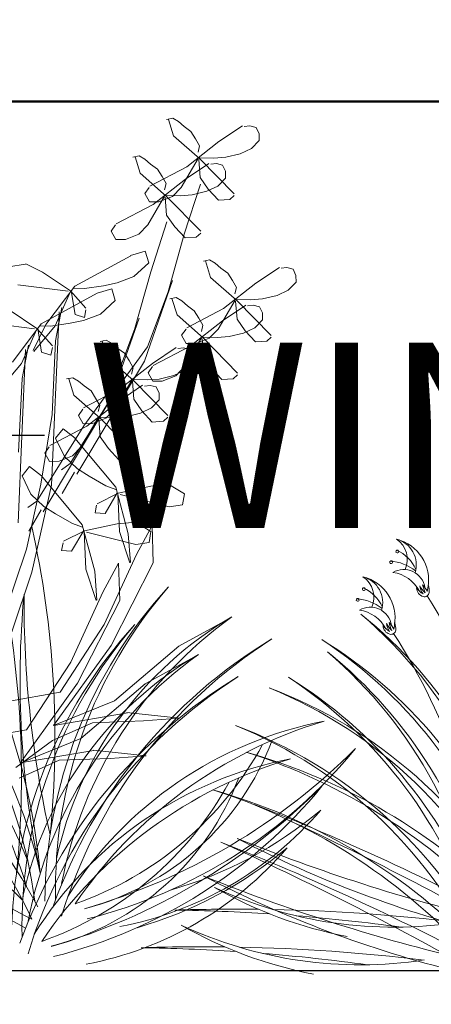
# Model space of a CAD drawing. Units: inches. Extents: x 89 to 490, y -59 to 378.
# Tile 9 of 20: x 339 to 352, y -24 to 7. Entities that reach past the tile are written whole.
import ezdxf

# ---------------------------------------------------------------- set-up
doc = ezdxf.new("R2010")
doc.units = ezdxf.units.IN
doc.header["$MEASUREMENT"] = 0
for name, color, linetype, lineweight in [('A-ANNO-DIMS', 2, 'Continuous', 18), ('L-PLNT', 94, 'Continuous', 18), ('L-PLNT-EDGE', 31, 'Continuous', 25), ('Outer Walls', 12, 'Continuous', 50), ('Windows', 171, 'Continuous', 25)]:
    doc.layers.add(name, color=color, linetype=linetype, lineweight=lineweight)
doc.layers.add('fl', color=73, linetype='Continuous', lineweight=9, true_color=0xa3d166)
doc.styles.get("Standard").update_dxf_attribs({"font": 'arial.ttf'})
doc.dimstyles.get("Standard").update_dxf_attribs({"dimtxt": 6, "dimasz": 4, "dimexe": 3, "dimexo": 3, "dimgap": 0.09, "dimtad": 0, "dimtih": 1, "dimtoh": 1, "dimdec": 1, "dimzin": 0, "dimdsep": 46, "dimlunit": 3, "dimtxsty": 'Standard', "dimcen": 0.09, "dimadec": 0, "dimazin": 0, "dimtfac": 1, "dimtdec": 1, "dimtofl": 0, "dimtmove": 0, "dimatfit": 3, "dimfxl": 1, "dimtolj": 1, "dimtzin": 0, "dimarcsym": 0})

# ---------------------------------------------------------------- blocks, each defined once
blk = doc.blocks.new('Window')
blk.add_lwpolyline([(588.369, 99.053), (588.369, 90.053), (516.369, 90.053), (516.369, 99.053)], close=True)
blk = doc.blocks.new('Plantation')
at = {"layer": 'fl'}
for p, q in [((567.452, 39.025), (567.652, 39.065)), ((567.52, 39.031), (567.683, 38.502)), ((567.652, 39.065), (567.835, 38.959)), ((567.835, 38.959), (568.02, 38.798)), ((568.02, 38.798), (568.241, 38.638)), ((568.241, 38.638), (568.391, 38.404)), ((569.148, 38.309), (569.909, 38.821)), ((570.148, 38.817), (569.967, 38.796)), ((570.349, 38.766), (570.148, 38.817)), ((570.444, 38.567), (570.349, 38.766)), ((570.448, 38.349), (570.444, 38.567)), ((567.683, 38.502), (568.535, 37.754)), ((568.107, 37.496), (569.148, 38.309)), ((568.391, 38.404), (568.522, 38.17)), ((570.198, 38.09), (570.448, 38.349)), ((568.522, 38.17), (568.471, 37.969)), ((569.366, 37.802), (569.837, 37.92)), ((569.837, 37.92), (570.198, 38.09)), ((566.368, 37.807), (566.568, 37.847)), ((566.436, 37.813), (566.6, 37.284)), ((566.568, 37.847), (566.752, 37.741)), ((566.752, 37.741), (566.936, 37.58)), ((567.927, 36.83), (568.475, 37.768)), ((568.065, 37.091), (568.825, 37.603)), ((568.494, 37.732), (568.54, 37.15)), ((568.529, 37.788), (568.984, 37.777)), ((568.535, 37.754), (569.643, 36.625)), ((569.065, 37.599), (568.883, 37.578)), ((568.984, 37.777), (569.366, 37.802)), ((569.266, 37.548), (569.065, 37.599)), ((566.6, 37.284), (567.452, 36.536)), ((566.913, 36.872), (568.107, 37.496)), ((566.936, 37.58), (567.157, 37.42)), ((567.157, 37.42), (567.307, 37.186)), ((569.36, 37.349), (569.266, 37.548)), ((569.364, 37.131), (569.36, 37.349)), ((567.023, 36.278), (568.065, 37.091)), ((567.307, 37.186), (567.439, 36.952)), ((568.54, 37.15), (568.801, 36.773)), ((569.114, 36.872), (569.364, 37.131)), ((566.89, 36.83), (566.748, 36.627)), ((567.439, 36.952), (567.387, 36.751)), ((567.641, 36.534), (567.927, 36.83)), ((568.024, 35.31), (568.552, 36.932)), ((568.282, 36.584), (568.753, 36.702)), ((568.753, 36.702), (569.114, 36.872)), ((568.801, 36.773), (569.135, 36.414)), ((566.748, 36.627), (566.898, 36.357)), ((566.843, 35.612), (567.391, 36.55)), ((566.898, 36.357), (567.208, 36.362)), ((567.208, 36.362), (567.641, 36.534)), ((567.41, 36.514), (567.456, 35.932)), ((567.445, 36.57), (567.9, 36.559)), ((567.452, 36.536), (568.56, 35.407)), ((567.9, 36.559), (568.282, 36.584)), ((569.135, 36.414), (569.499, 36.439)), ((569.499, 36.439), (569.642, 36.569)), ((565.829, 35.654), (567.023, 36.278)), ((566.94, 34.092), (567.468, 35.714)), ((567.456, 35.932), (567.718, 35.555)), ((565.806, 35.612), (565.664, 35.409)), ((565.664, 35.409), (565.815, 35.139)), ((566.557, 35.316), (566.843, 35.612)), ((567.718, 35.555), (568.051, 35.196)), ((565.815, 35.139), (566.124, 35.144)), ((566.124, 35.144), (566.557, 35.316)), ((567.504, 33.445), (568.024, 35.31)), ((568.051, 35.196), (568.415, 35.221)), ((568.415, 35.221), (568.558, 35.351)), ((566.767, 34.761), (566.292, 34.62)), ((566.88, 34.391), (566.767, 34.761)), ((564.484, 33.634), (566.297, 34.619)), ((568.645, 34.441), (568.845, 34.481)), ((568.713, 34.447), (568.877, 33.918)), ((568.845, 34.481), (569.029, 34.375)), ((562.897, 34.348), (562.341, 34.259)), ((562.903, 34.358), (563.447, 34.084)), ((566.397, 33.944), (566.88, 34.391)), ((566.42, 32.227), (566.94, 34.092)), ((569.029, 34.375), (569.213, 34.214)), ((569.213, 34.214), (569.435, 34.054)), ((570.342, 33.725), (571.102, 34.237)), ((571.342, 34.233), (571.16, 34.212)), ((571.543, 34.182), (571.342, 34.233)), ((571.637, 33.983), (571.543, 34.182)), ((563.447, 34.084), (564.343, 33.483)), ((565.856, 33.736), (566.397, 33.944)), ((566.737, 31.205), (567.647, 33.818)), ((568.877, 33.918), (569.729, 33.169)), ((569.435, 34.054), (569.584, 33.82)), ((569.584, 33.82), (569.716, 33.586)), ((571.641, 33.765), (571.637, 33.983)), ((562.643, 33.679), (564.267, 33.469)), ((563.554, 32.387), (564.484, 33.634)), ((563.848, 32.345), (564.347, 33.457)), ((564.343, 33.483), (564.848, 32.917)), ((564.493, 32.715), (564.373, 33.484)), ((564.451, 33.565), (564.797, 33.558)), ((564.797, 33.558), (565.419, 33.648)), ((565.683, 33.543), (565.208, 33.402)), ((565.419, 33.648), (565.856, 33.736)), ((565.796, 33.173), (565.683, 33.543)), ((569.3, 32.912), (570.342, 33.725)), ((569.716, 33.586), (569.665, 33.384)), ((571.03, 33.335), (571.391, 33.505)), ((571.391, 33.505), (571.641, 33.765)), ((563.4, 32.416), (565.213, 33.401)), ((565.313, 32.726), (565.796, 33.173)), ((566.835, 31.672), (567.504, 33.445)), ((567.562, 33.223), (567.761, 33.263)), ((567.629, 33.229), (567.793, 32.7)), ((567.761, 33.263), (567.945, 33.157)), ((567.945, 33.157), (568.13, 32.996)), ((569.12, 32.246), (569.668, 33.184)), ((569.687, 33.148), (569.733, 32.566)), ((569.722, 33.203), (570.177, 33.193)), ((569.729, 33.169), (570.837, 32.04)), ((570.177, 33.193), (570.559, 33.218)), ((570.559, 33.218), (571.03, 33.335)), ((562.363, 32.866), (563.259, 32.265)), ((563.863, 31.862), (564.07, 32.939)), ((564.848, 32.868), (564.8, 32.614)), ((568.106, 32.288), (569.3, 32.912)), ((568.13, 32.996), (568.351, 32.836)), ((568.351, 32.836), (568.5, 32.602)), ((569.258, 32.507), (570.018, 33.019)), ((570.258, 33.015), (570.076, 32.994)), ((570.459, 32.964), (570.258, 33.015)), ((570.553, 32.765), (570.459, 32.964)), ((563.978, 32.797), (563.734, 27.189)), ((564.335, 32.43), (564.772, 32.518)), ((564.8, 32.614), (564.493, 32.715)), ((564.772, 32.518), (565.313, 32.726)), ((565.653, 29.987), (566.564, 32.6)), ((567.793, 32.7), (568.645, 31.951)), ((568.216, 31.694), (569.258, 32.507)), ((568.5, 32.602), (568.632, 32.367)), ((569.733, 32.566), (569.995, 32.188)), ((570.307, 32.287), (570.557, 32.547)), ((570.557, 32.547), (570.553, 32.765)), ((561.559, 32.461), (563.183, 32.251)), ((562.47, 31.169), (563.4, 32.416)), ((562.765, 31.127), (563.263, 32.239)), ((563.145, 31.546), (563.554, 32.387)), ((563.159, 31.523), (563.848, 32.345)), ((563.259, 32.265), (563.764, 31.699)), ((563.409, 31.497), (563.289, 32.266)), ((563.367, 32.347), (563.713, 32.34)), ((563.713, 32.34), (564.335, 32.43)), ((565.751, 30.454), (566.42, 32.227)), ((568.083, 32.246), (567.941, 32.043)), ((568.632, 32.367), (568.581, 32.166)), ((568.834, 31.95), (569.12, 32.246)), ((569.946, 32.117), (570.307, 32.287)), ((569.995, 32.188), (570.328, 31.83)), ((563.75, 29.477), (563.863, 31.862)), ((565.306, 31.847), (565.506, 31.887)), ((565.506, 31.887), (565.69, 31.781)), ((567.941, 32.043), (568.092, 31.773)), ((568.037, 31.028), (568.584, 31.966)), ((568.401, 31.778), (568.834, 31.95)), ((568.603, 31.93), (568.65, 31.348)), ((568.638, 31.985), (569.093, 31.975)), ((568.645, 31.951), (569.753, 30.822)), ((569.093, 31.975), (569.475, 32)), ((569.475, 32), (569.946, 32.117)), ((570.692, 31.855), (570.835, 31.984)), ((562.894, 31.579), (562.65, 25.971)), ((562.78, 30.644), (562.986, 31.721)), ((563.765, 31.65), (563.716, 31.396)), ((565.374, 31.853), (565.537, 31.324)), ((565.69, 31.781), (565.874, 31.62)), ((565.86, 30.326), (566.835, 31.672)), ((565.874, 31.62), (566.095, 31.46)), ((567.002, 31.131), (567.763, 31.643)), ((567.022, 31.07), (568.216, 31.694)), ((568.002, 31.639), (567.821, 31.618)), ((568.203, 31.588), (568.002, 31.639)), ((568.092, 31.773), (568.401, 31.778)), ((568.298, 31.389), (568.203, 31.588)), ((570.328, 31.83), (570.692, 31.855)), ((563.716, 31.396), (563.409, 31.497)), ((565.537, 31.324), (566.389, 30.575)), ((566.095, 31.46), (566.245, 31.226)), ((566.245, 31.226), (566.376, 30.992)), ((568.302, 31.171), (568.298, 31.389)), ((568.65, 31.348), (568.911, 30.97)), ((562.075, 30.305), (562.765, 31.127)), ((564.547, 27.545), (566.737, 31.205)), ((565.961, 30.318), (567.002, 31.131)), ((566.376, 30.992), (566.325, 30.79)), ((567, 31.028), (566.858, 30.825)), ((567.691, 30.741), (568.052, 30.912)), ((567.751, 30.732), (568.037, 31.028)), ((568.052, 30.912), (568.302, 31.171)), ((568.911, 30.97), (569.245, 30.612)), ((562.666, 28.259), (562.78, 30.644)), ((564.222, 30.629), (564.422, 30.669)), ((564.29, 30.635), (564.454, 30.106)), ((564.422, 30.669), (564.606, 30.563)), ((565.781, 29.652), (566.329, 30.59)), ((566.383, 30.609), (566.838, 30.599)), ((566.838, 30.599), (567.22, 30.624)), ((566.858, 30.825), (567.008, 30.555)), ((567.22, 30.624), (567.691, 30.741)), ((567.317, 30.56), (567.751, 30.732)), ((569.245, 30.612), (569.608, 30.637)), ((569.608, 30.637), (569.751, 30.766)), ((564.339, 27.892), (565.86, 30.326)), ((564.606, 30.563), (564.79, 30.402)), ((564.767, 29.694), (565.961, 30.318)), ((564.776, 29.108), (565.751, 30.454)), ((564.79, 30.402), (565.012, 30.242)), ((565.919, 29.913), (566.679, 30.425)), ((566.348, 30.554), (566.394, 29.972)), ((566.389, 30.575), (567.497, 29.447)), ((566.919, 30.421), (566.737, 30.4)), ((567.12, 30.37), (566.919, 30.421)), ((567.008, 30.555), (567.317, 30.56)), ((567.214, 30.171), (567.12, 30.37)), ((563.463, 26.327), (565.653, 29.987)), ((564.454, 30.106), (565.306, 29.357)), ((565.012, 30.242), (565.161, 30.008)), ((565.161, 30.008), (565.293, 29.774)), ((566.394, 29.972), (566.656, 29.594)), ((566.968, 29.694), (567.218, 29.953)), ((567.218, 29.953), (567.214, 30.171)), ((564.744, 29.652), (564.602, 29.449)), ((564.877, 29.1), (565.919, 29.913)), ((565.293, 29.774), (565.242, 29.572)), ((565.495, 29.356), (565.781, 29.652)), ((566.607, 29.523), (566.968, 29.694)), ((563.389, 27.228), (563.75, 29.477)), ((564.602, 29.449), (564.753, 29.179)), ((564.697, 28.434), (565.245, 29.372)), ((565.062, 29.184), (565.495, 29.356)), ((565.264, 29.336), (565.31, 28.754)), ((565.299, 29.391), (565.754, 29.381)), ((565.306, 29.357), (566.414, 28.229)), ((565.754, 29.381), (566.136, 29.406)), ((566.136, 29.406), (566.607, 29.523)), ((566.656, 29.594), (566.989, 29.236)), ((567.353, 29.261), (567.496, 29.391)), ((563.255, 26.674), (564.776, 29.108)), ((563.683, 28.476), (564.877, 29.1)), ((563.864, 28.713), (564.105, 29.016)), ((564.105, 29.016), (564.495, 28.709)), ((564.753, 29.179), (565.062, 29.184)), ((566.989, 29.236), (567.353, 29.261)), ((564.148, 28.119), (563.864, 28.713)), ((565.812, 27.125), (564.489, 28.71)), ((565.31, 28.754), (565.572, 28.376)), ((563.66, 28.434), (563.518, 28.231)), ((564.412, 28.138), (564.697, 28.434)), ((565.572, 28.376), (565.905, 28.018)), ((563.518, 28.231), (563.669, 27.961)), ((563.978, 27.966), (564.412, 28.138)), ((564.574, 27.726), (564.148, 28.119)), ((565.905, 28.018), (566.269, 28.043)), ((566.269, 28.043), (566.412, 28.173)), ((562.78, 27.495), (563.021, 27.798)), ((563.021, 27.798), (563.411, 27.491)), ((563.669, 27.961), (563.978, 27.966)), ((564.054, 27.688), (564.339, 27.892)), ((564.948, 27.484), (564.574, 27.726)), ((563.064, 26.901), (562.78, 27.495)), ((564.728, 25.907), (563.405, 27.492)), ((564.08, 26.921), (564.478, 27.612)), ((565.493, 27.17), (564.948, 27.484)), ((562.927, 25.122), (563.389, 27.228)), ((563.734, 27.189), (563.1, 24.376)), ((565.817, 27.05), (565.493, 27.17)), ((566.216, 25.623), (565.812, 27.125)), ((566.941, 27.162), (565.887, 26.933)), ((567.548, 27.216), (566.941, 27.162)), ((567.55, 27.205), (568.034, 26.917)), ((563.49, 26.508), (563.064, 26.901)), ((565.887, 26.933), (565.209, 26.594)), ((565.465, 26.275), (565.86, 26.945)), ((565.927, 25.693), (565.874, 26.911)), ((567.539, 26.49), (565.952, 26.892)), ((568.034, 26.917), (567.97, 26.555)), ((562.97, 26.47), (563.255, 26.674)), ((563.864, 26.266), (563.49, 26.508)), ((565.19, 26.548), (565.142, 26.294)), ((567.97, 26.555), (567.539, 26.49)), ((562.996, 25.703), (563.394, 26.394)), ((564.409, 25.952), (563.864, 26.266)), ((565.142, 26.294), (565.465, 26.275)), ((564.733, 25.832), (564.409, 25.952)), ((565.133, 24.405), (564.728, 25.907)), ((565.858, 25.944), (564.803, 25.715)), ((566.464, 25.998), (565.858, 25.944)), ((566.466, 25.987), (566.95, 25.699)), ((566.481, 24.951), (566.984, 25.892)), ((566.984, 25.892), (567.025, 24.678)), ((564.803, 25.715), (564.125, 25.376)), ((564.381, 25.057), (564.776, 25.727)), ((564.844, 24.475), (564.79, 25.693)), ((566.456, 25.272), (564.869, 25.674)), ((566.265, 24.675), (565.927, 25.693)), ((566.287, 24.692), (566.216, 25.623)), ((566.95, 25.699), (566.886, 25.337)), ((564.106, 25.33), (564.058, 25.076)), ((566.886, 25.337), (566.456, 25.272)), ((562.176, 22.909), (562.927, 25.122)), ((564.058, 25.076), (564.381, 25.057)), ((565.44, 22.68), (566.481, 24.951)), ((565.397, 23.733), (565.9, 24.674)), ((567.025, 24.678), (565.658, 22.007)), ((565.9, 24.674), (565.941, 23.46)), ((563.1, 24.376), (562.451, 22.451)), ((565.181, 23.457), (564.844, 24.475)), ((565.203, 23.474), (565.133, 24.405)), ((564.357, 21.462), (565.397, 23.733)), ((565.941, 23.46), (564.574, 20.789)), ((564.008, 20.492), (565.44, 22.68)), ((567.846, 21.984), (569.564, 22.918)), ((565.658, 22.007), (563.802, 19.415)), ((565.768, 20.212), (567.846, 21.984)), ((566.762, 20.766), (568.481, 21.7)), ((562.924, 19.274), (564.357, 21.462)), ((564.574, 20.789), (562.718, 18.197)), ((564.684, 18.994), (566.762, 20.766)), ((562.317, 20.191), (564.008, 20.492)), ((563.802, 19.415), (565.768, 20.212)), ((566.19, 19.825), (563.803, 19.421)), ((566.169, 19.836), (567.877, 19.652)), ((565.063, 19.507), (563.77, 18.928)), ((566.713, 19.563), (565.063, 19.507)), ((567.877, 19.652), (566.713, 19.563)), ((561.233, 18.973), (562.924, 19.274)), ((563.77, 18.928), (562.584, 18.061)), ((562.718, 18.197), (564.684, 18.994)), ((565.106, 18.607), (562.719, 18.203)), ((565.086, 18.618), (566.793, 18.434)), ((563.979, 18.289), (562.686, 17.71)), ((565.63, 18.345), (563.979, 18.289)), ((566.793, 18.434), (565.63, 18.345))]:
    blk.add_line(p, q, dxfattribs=at)
for centre, radius, start, end in [((532.353, 19.019), 31.492, 354.2791, 12.5427), ((574.665, 24.613), 0.863, 342.816, 75.0201), ((574.448, 24.787), 0.793, 335.7976, 56.2278), ((574.561, 24.118), 1.368, 349.633, 76.1366), ((574.916, 25.045), 0.0459, 19.649, 199.649), ((574.916, 25.045), 0.0459, 199.649, 19.649), ((574.381, 23.96), 1.243, 24.0842, 65.3008), ((531.269, 17.801), 31.492, 354.2791, 12.5427), ((574.717, 24.698), 0.0459, 19.649, 199.649), ((574.717, 24.698), 0.0459, 199.649, 19.649), ((574.622, 23.348), 1.386, 50.416, 87.3549), ((573.582, 23.395), 0.863, 342.816, 75.0201), ((573.364, 23.569), 0.793, 335.7976, 56.2278), ((573.477, 22.9), 1.368, 349.633, 76.1366), ((575.124, 23.766), 0.696, 9.2042, 120.225), ((574.609, 23.226), 1.154, 27.9293, 81.8071), ((578.721, 13.629), 15.201, 137.4916, 179.6099), ((578.783, 14.119), 14.921, 139.0392, 181.297), ((576.209, 24.004), 0.565, 186.5701, 215.6042), ((576.311, 24.251), 0.733, 205.1582, 227.5978), ((575.252, 23.466), 0.694, 24.1932, 45.802), ((577.016, 24.232), 1.308, 191.8611, 203.5164), ((574.864, 23.987), 1.049, 346.9198, 358.7337), ((575.354, 23.758), 0.595, 356.0005, 20.2804), ((543.232, 12.838), 20.216, 5.151, 32.7872), ((592.609, 20.863), 29.894, 174.6174, 191.9895), ((596.834, 23.399), 33.989, 179.5471, 192.7817), ((573.832, 23.827), 0.0459, 19.649, 199.649), ((573.832, 23.827), 0.0459, 199.649, 19.649), ((573.297, 22.742), 1.243, 24.0842, 65.3008), ((575.831, 23.868), 0.289, 180.2252, 254.4537), ((576.039, 24.197), 0.596, 213.5892, 240.9815), ((575.798, 23.734), 0.151, 253.2058, 353.1709), ((558.885, 12.66), 20.216, 5.151, 32.7872), ((573.633, 23.48), 0.0459, 19.649, 199.649), ((573.633, 23.48), 0.0459, 199.649, 19.649), ((573.538, 22.13), 1.386, 50.416, 87.3549), ((548.387, 11.862), 14.921, 7.1968, 49.4547), ((548.521, 11.386), 15.201, 12.4122, 51.0023), ((574.04, 22.548), 0.696, 9.2042, 120.225), ((573.525, 22.008), 1.154, 27.9293, 81.8071), ((564.04, 11.683), 14.921, 7.1968, 49.4547), ((564.174, 11.208), 15.201, 12.4122, 51.0023), ((577.637, 12.411), 15.201, 137.4916, 179.6099), ((577.699, 12.901), 14.921, 139.0392, 181.297), ((575.641, 12.566), 12.017, 120.3536, 167.8423), ((577.67, 11.695), 13.856, 125.7805, 169.1581), ((574.748, 22.65), 0.289, 180.2252, 254.4537), ((574.955, 22.979), 0.596, 213.5892, 240.9815), ((575.125, 22.786), 0.565, 186.5701, 215.6042), ((575.228, 23.033), 0.733, 205.1582, 227.5978), ((574.169, 22.247), 0.694, 24.1932, 45.802), ((575.933, 23.014), 1.308, 191.8611, 203.5164), ((573.78, 22.769), 1.049, 346.9198, 358.7337), ((574.271, 22.54), 0.595, 356.0005, 20.2804), ((548.639, 9.896), 14.921, 16.8321, 56.7339), ((548.831, 9.441), 15.201, 21.5651, 58.2814), ((574.714, 22.516), 0.151, 253.2058, 353.1709), ((557.801, 11.442), 20.216, 5.151, 32.7872), ((579.464, 7.974), 16.642, 121.1471, 160.292), ((579.598, 8.531), 16.239, 122.567, 163.1344), ((564.292, 9.718), 14.921, 16.8321, 56.7339), ((564.484, 9.263), 15.201, 21.5651, 58.2814), ((574.557, 11.348), 12.017, 120.3536, 167.8423), ((576.586, 10.477), 13.856, 125.7805, 169.1581), ((562.957, 10.465), 14.921, 7.1968, 49.4547), ((563.09, 9.99), 15.201, 12.4122, 51.0023), ((549.776, 6.58), 15.201, 27.2807, 69.4256), ((549.5, 6.989), 14.921, 24.3637, 67.878), ((578.381, 6.756), 16.642, 121.1471, 160.292), ((578.514, 7.313), 16.239, 122.567, 163.1344), ((563.208, 8.5), 14.921, 16.8321, 56.7339), ((563.401, 8.045), 15.201, 21.5651, 58.2814), ((565.43, 6.402), 15.201, 27.2807, 69.4256), ((565.153, 6.811), 14.921, 24.3637, 67.878), ((574.953, 7.146), 12.64, 100.96, 147.8088), ((576.837, 5.275), 14.911, 106.7083, 145.8338), ((564.346, 5.184), 15.201, 27.2807, 69.4256), ((564.069, 5.593), 14.921, 24.3637, 67.878), ((560.859, 24.074), 11.042, 289.2472, 331.4766), ((562.565, 22.08), 8.88, 284.6053, 339.2893), ((549.158, 0.259), 19.194, 44.7494, 74.2143), ((559.09, 33.14), 20.466, 286.2137, 315.0057), ((560.915, 28.99), 16.324, 284.0723, 320.7861), ((564.812, 0.081), 19.194, 44.7494, 74.2143), ((564.189, 0.318), 19.147, 42.8064, 72.2288), ((573.869, 5.928), 12.64, 100.96, 147.8088), ((575.753, 4.057), 14.911, 106.7083, 145.8338), ((559.776, 22.856), 11.042, 289.2472, 331.4766), ((561.481, 20.862), 8.88, 284.6053, 339.2893), ((558.006, 31.922), 20.466, 286.2137, 315.0057), ((559.832, 27.772), 16.324, 284.0723, 320.7861), ((563.728, -1.137), 19.194, 44.7494, 74.2143), ((563.105, -0.9), 19.147, 42.8064, 72.2288), ((510.112, -81.018), 107.696, 60.65352, 65.57668), ((524.246, -59.986), 82.807, 62.02355, 68.46556), ((563.829, 24.037), 11.325, 280.7497, 319.4803), ((563.965, 26.719), 13.137, 285.9859, 310.1616), ((525.765, -81.196), 107.696, 60.65352, 65.57668), ((539.899, -60.164), 82.807, 62.02355, 68.46556), ((524.681, -82.414), 107.696, 60.65352, 65.57668), ((538.815, -61.382), 82.807, 62.02355, 68.46556), ((586.697, 48.387), 36.77, 242.5259, 256.2554), ((591.684, 70.033), 58.541, 247.9781, 256.44), ((562.745, 22.819), 11.325, 280.7497, 319.4803), ((562.881, 25.501), 13.137, 285.9859, 310.1616), ((585.614, 47.169), 36.77, 242.5259, 256.2554), ((590.6, 68.815), 58.541, 247.9781, 256.44), ((575.964, 26.375), 14.044, 240.3144, 259.0249), ((574.803, 26.594), 13.704, 244.9915, 278.6666), ((569.681, -46.882), 60.356, 89.2944, 91.86186), ((566.848, -46.949), 60.398, 86.26075, 89.17238), ((569.681, -46.882), 60.356, 83.15791, 88.86091), ((566.848, -46.949), 60.398, 82.20958, 85.44376), ((574.88, 25.157), 14.044, 240.3144, 259.0249), ((573.719, 25.376), 13.704, 244.9915, 278.6666), ((568.598, -48.1), 60.356, 89.2944, 91.86186), ((565.764, -48.167), 60.398, 86.26075, 89.17238), ((568.598, -48.1), 60.356, 83.15791, 88.86091), ((565.764, -48.167), 60.398, 82.20958, 85.44376)]:
    blk.add_arc(centre, radius, start, end, dxfattribs=at)
blk = doc.blocks.new('*D36')
at = {"layer": 'A-ANNO-DIMS', "color": 0, "lineweight": -2, "transparency": 16777216}
for p, q in [((327.654, 1.741), (327.654, -9.059)), ((399.654, 1.741), (399.654, -9.059)), ((331.654, -6.059), (339.621, -6.059)), ((395.654, -6.059), (387.687, -6.059))]:
    blk.add_line(p, q, dxfattribs=at)
at = {"layer": 'A-ANNO-DIMS', "color": 0, "transparency": 16777216}
for points in [[(331.654, -5.392), (331.654, -6.725), (327.654, -6.059)], [(395.654, -5.392), (395.654, -6.725), (399.654, -6.059)]]:
    blk.add_solid(points, dxfattribs=at)
at = {"layer": 'Defpoints', "color": 0, "transparency": 16777216}
for p in [(327.654, 4.741), (399.654, 4.741), (399.654, -6.059)]:
    blk.add_point(p, dxfattribs=at)
at = {"layer": 'A-ANNO-DIMS', "color": 0, "transparency": 16777216, "insert": (363.654, -6.059), "char_height": 6, "attachment_point": 5}
blk.add_mtext('\\A1;WINDOW 72', dxfattribs=at)
blk = doc.blocks.new('*D48')
at = {"layer": 'A-ANNO-DIMS', "color": 0, "lineweight": -2, "transparency": 16777216}
for p, q in [((127.441, 10.741), (127.441, -49.809)), ((459.441, -29.659), (459.441, -49.809)), ((131.441, -46.809), (286.756, -46.809)), ((455.441, -46.809), (300.127, -46.809))]:
    blk.add_line(p, q, dxfattribs=at)
at = {"layer": 'A-ANNO-DIMS', "color": 0, "transparency": 16777216}
for points in [[(131.441, -46.143), (131.441, -47.476), (127.441, -46.809)], [(455.441, -46.143), (455.441, -47.476), (459.441, -46.809)]]:
    blk.add_solid(points, dxfattribs=at)
at = {"layer": 'Defpoints', "color": 0, "transparency": 16777216}
for p in [(127.441, 13.741), (459.441, -26.659), (459.441, -46.809)]:
    blk.add_point(p, dxfattribs=at)
at = {"layer": 'A-ANNO-DIMS', "color": 0, "transparency": 16777216, "insert": (293.441, -46.809), "char_height": 6, "attachment_point": 5}
blk.add_mtext('\\A1;332', dxfattribs=at)

msp = doc.modelspace()

# ---------------------------------------------------------------- linework, layer by layer
at = {"layer": 'L-PLNT-EDGE'}
msp.add_line((459.4414, -23.3886), (265.4414, -23.3886), dxfattribs=at)
at = {"layer": 'Outer Walls'}
msp.add_lwpolyline([(214.6478, 67.7413), (265.4414, 67.7413), (265.4414, 4.7413), (459.4414, 4.7413), (459.4414, 353.7413), (127.4414, 353.7413), (127.4414, 13.7413)], dxfattribs=at)

# ---------------------------------------------------------------- block references
at = {"layer": 'L-PLNT'}
msp.add_blockref('Plantation', (-223.8856, -34.8668), dxfattribs=at)
at = {"layer": 'Windows'}
msp.add_blockref('Window', (-188.7147, -85.3119), dxfattribs=at)

# ---------------------------------------------------------------- dimensions: what is measured, and where the dimension line sits
at = {"layer": 'A-ANNO-DIMS'}
dim = msp.add_linear_dim(base=(459.4414, -46.8094), p1=(127.4414, 13.7413), p2=(459.4414, -26.6594), dimstyle='Standard', override={"dimdec": 0, "dimlfac": 1, "dimrnd": 0, "dimzin": 0, "dimdsep": 46, "dimlunit": 2}, dxfattribs=at)
dim.commit()
dim.dimension.update_dxf_attribs({"geometry": '*D48', "text_midpoint": (293.4414, -46.8094)})
dim = msp.add_linear_dim(base=(399.6539, -6.0587), p1=(327.6539, 4.7413), p2=(399.6539, 4.7413), text='WINDOW <>', dimstyle='Standard', override={"dimdec": 0, "dimlfac": 1, "dimrnd": 0, "dimzin": 0, "dimdsep": 46, "dimlunit": 2}, dxfattribs=at)
dim.commit()
dim.dimension.update_dxf_attribs({"geometry": '*D36', "text_midpoint": (363.6539, -6.0587)})

doc.saveas('drawing.dxf')
